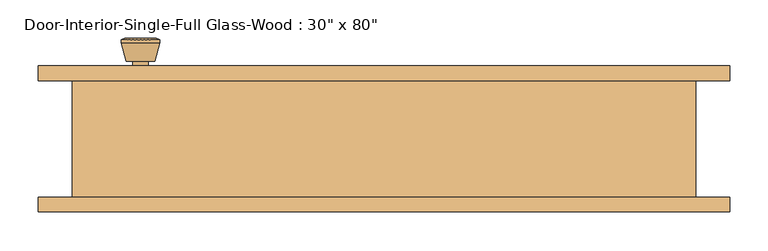
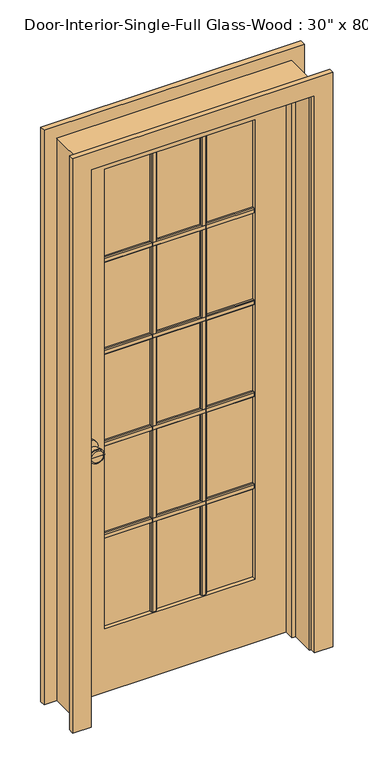
"""IFC4 building model written with IfcOpenShell, lengths in millimetres: door geometry."""

from ifc_helpers import new_model, si_unit, point, frame, frame_2d, origin, place, context, project, spatial, polyline, circle_curve, trimmed, segment, composite_curve, outline, extrude, faceted_brep, source, transform, mapped, element, save
from ifc_brep_helpers import plane_surface, cylinder_surface, revolved_surface, advanced_brep


def door_fa41f557(model_context):
    return source(origin(), model_context, "Body", "SolidModel", [
        extrude(outline(polyline([(59.055, 1586.23), (65.405, 1586.23), (68.58, 1583.055), (68.58, 1570.355), (65.405, 1567.18), (59.055, 1567.18), (59.055, 1586.23)])), frame((-260.35, 0.0, 0.0), z_axis=(1.0, 0.0, 0.0), x_axis=(0.0, 1.0, 0.0)), (0.0, 0.0, 1.0), 520.7),
        extrude(outline(polyline([(59.055, 1249.9975), (65.405, 1249.9975), (68.58, 1246.8225), (68.58, 1234.1225), (65.405, 1230.9475), (59.055, 1230.9475), (59.055, 1249.9975)])), frame((-260.35, 0.0, 0.0), z_axis=(1.0, 0.0, 0.0), x_axis=(0.0, 1.0, 0.0)), (0.0, 0.0, 1.0), 520.7),
        extrude(outline(polyline([(59.055, 913.765), (65.405, 913.765), (68.58, 910.59), (68.58, 897.89), (65.405, 894.715), (59.055, 894.715), (59.055, 913.765)])), frame((-260.35, 0.0, 0.0), z_axis=(1.0, 0.0, 0.0), x_axis=(0.0, 1.0, 0.0)), (0.0, 0.0, 1.0), 520.7),
        extrude(outline(polyline([(59.055, 577.5325), (65.405, 577.5325), (68.58, 574.3575), (68.58, 561.6575), (65.405, 558.4825), (59.055, 558.4825), (59.055, 577.5325)])), frame((-260.35, 0.0, 0.0), z_axis=(1.0, 0.0, 0.0), x_axis=(0.0, 1.0, 0.0)), (0.0, 0.0, 1.0), 520.7),
        extrude(outline(polyline([(77.2583333, 59.055), (77.2583333, 65.405), (80.4333333, 68.58), (93.1333333, 68.58), (96.3083333, 65.405), (96.3083333, 59.055), (77.2583333, 59.055)])), frame((0.0, 0.0, 231.775), z_axis=(0.0, 0.0, 1.0), x_axis=(1.0, 0.0, 0.0)), (0.0, 0.0, 1.0), 1681.1625),
        extrude(outline(polyline([(-96.3083333, 59.055), (-96.3083333, 65.405), (-93.1333333, 68.58), (-80.4333333, 68.58), (-77.2583333, 65.405), (-77.2583333, 59.055), (-96.3083333, 59.055)])), frame((0.0, 0.0, 231.775), z_axis=(0.0, 0.0, 1.0), x_axis=(1.0, 0.0, 0.0)), (0.0, 0.0, 1.0), 1681.1625),
        extrude(outline(polyline([(52.07, 1586.23), (52.07, 1567.18), (45.72, 1567.18), (42.545, 1570.355), (42.545, 1583.055), (45.72, 1586.23), (52.07, 1586.23)])), frame((-260.35, 0.0, 0.0), z_axis=(1.0, 0.0, 0.0), x_axis=(0.0, 1.0, 0.0)), (0.0, 0.0, 1.0), 520.7),
        extrude(outline(polyline([(52.07, 1249.9975), (52.07, 1230.9475), (45.72, 1230.9475), (42.545, 1234.1225), (42.545, 1246.8225), (45.72, 1249.9975), (52.07, 1249.9975)])), frame((-260.35, 0.0, 0.0), z_axis=(1.0, 0.0, 0.0), x_axis=(0.0, 1.0, 0.0)), (0.0, 0.0, 1.0), 520.7),
        extrude(outline(polyline([(52.07, 913.765), (52.07, 894.715), (45.72, 894.715), (42.545, 897.89), (42.545, 910.59), (45.72, 913.765), (52.07, 913.765)])), frame((-260.35, 0.0, 0.0), z_axis=(1.0, 0.0, 0.0), x_axis=(0.0, 1.0, 0.0)), (0.0, 0.0, 1.0), 520.7),
        extrude(outline(polyline([(52.07, 577.5325), (52.07, 558.4825), (45.72, 558.4825), (42.545, 561.6575), (42.545, 574.3575), (45.72, 577.5325), (52.07, 577.5325)])), frame((-260.35, 0.0, 0.0), z_axis=(1.0, 0.0, 0.0), x_axis=(0.0, 1.0, 0.0)), (0.0, 0.0, 1.0), 520.7),
        extrude(outline(polyline([(77.2583333, 52.07), (96.3083333, 52.07), (96.3083333, 45.72), (93.1333333, 42.545), (80.4333333, 42.545), (77.2583333, 45.72), (77.2583333, 52.07)])), frame((0.0, 0.0, 231.775), z_axis=(0.0, 0.0, 1.0), x_axis=(1.0, 0.0, 0.0)), (0.0, 0.0, 1.0), 1681.1625),
        extrude(outline(polyline([(-96.3083333, 52.07), (-77.2583333, 52.07), (-77.2583333, 45.72), (-80.4333333, 42.545), (-93.1333333, 42.545), (-96.3083333, 45.72), (-96.3083333, 52.07)])), frame((0.0, 0.0, 231.775), z_axis=(0.0, 0.0, 1.0), x_axis=(1.0, 0.0, 0.0)), (0.0, 0.0, 1.0), 1681.1625),
        advanced_brep(
        [(-317.5, 32.1, 914.4), (-307.5, 32.1, 914.4), (-327.5, 32.1, 914.4), (-297.0241324, -16.9, 914.4), (-317.5, -16.9, 914.4), (-337.9758676, -16.9, 914.4), (-292.5, -15.0721319, 914.4), (-342.5, -15.0721319, 914.4), (-292.5, -11.6084537, 914.4), (-342.5, -11.6084537, 914.4), (-298.863764, 13.1, 914.4), (-336.136236, 13.1, 914.4), (-307.5, 13.1, 914.4), (-327.5, 13.1, 914.4)],
        [
            (0, 1),
            (1, 2, circle_curve(frame((-317.5, 32.1, 914.4), z_axis=(0.0, 1.0, 0.0), x_axis=(-1.0, 0.0, 0.0)), 10.0)),
            (2, 0),
            (2, 1, circle_curve(frame((-317.5, 32.1, 914.4), z_axis=(0.0, 1.0, 0.0), x_axis=(-1.0, 0.0, 0.0)), 10.0)),
            (3, 4),
            (4, 5),
            (5, 3, circle_curve(frame((-317.5, -16.9, 914.4), z_axis=(0.0, -1.0, 0.0), x_axis=(-1.0, 0.0, 0.0)), 20.4758676)),
            (3, 5, circle_curve(frame((-317.5, -16.9, 914.4), z_axis=(0.0, -1.0, 0.0), x_axis=(-1.0, 0.0, 0.0)), 20.4758676)),
            (6, 3),
            (5, 7),
            (7, 6, circle_curve(frame((-317.5, -15.0721319, 914.4), z_axis=(0.0, -1.0, 0.0), x_axis=(-1.0, 0.0, 0.0)), 25.0)),
            (6, 7, circle_curve(frame((-317.5, -15.0721319, 914.4), z_axis=(0.0, -1.0, 0.0), x_axis=(-1.0, 0.0, 0.0)), 25.0)),
            (8, 6),
            (7, 9),
            (9, 8, circle_curve(frame((-317.5, -11.6084537, 914.4), z_axis=(0.0, -1.0, 0.0), x_axis=(-1.0, 0.0, 0.0)), 25.0)),
            (8, 9, circle_curve(frame((-317.5, -11.6084537, 914.4), z_axis=(0.0, -1.0, 0.0), x_axis=(-1.0, 0.0, 0.0)), 25.0)),
            (10, 8),
            (9, 11),
            (11, 10, circle_curve(frame((-317.5, 13.1, 914.4), z_axis=(0.0, -1.0, 0.0), x_axis=(-1.0, 0.0, 0.0)), 18.636236)),
            (10, 11, circle_curve(frame((-317.5, 13.1, 914.4), z_axis=(0.0, -1.0, 0.0), x_axis=(-1.0, 0.0, 0.0)), 18.636236)),
            (12, 10),
            (11, 13),
            (13, 12, circle_curve(frame((-317.5, 13.1, 914.4), z_axis=(0.0, -1.0, 0.0), x_axis=(-1.0, 0.0, 0.0)), 10.0)),
            (12, 13, circle_curve(frame((-317.5, 13.1, 914.4), z_axis=(0.0, -1.0, 0.0), x_axis=(-1.0, 0.0, 0.0)), 10.0)),
            (1, 12),
            (13, 2),
        ],
        [
            plane_surface(frame((-317.5, 32.1, 914.4), z_axis=(0.0, 1.0, 0.0), x_axis=(-1.0, 0.0, 0.0))),
            plane_surface(frame((-317.5, -16.9, 914.4), z_axis=(0.0, -1.0, 0.0), x_axis=(-1.0, 0.0, 0.0))),
            revolved_surface(polyline([(-337.9758676, -16.9, 914.4), (-342.5, -15.0721319, 914.4)]), (-317.5, 32.1, 914.4), (0.0, 1.0, 0.0)),
            cylinder_surface(frame((-317.5, 32.1, 914.4), z_axis=(0.0, 1.0, 0.0), x_axis=(-1.0, 0.0, 0.0)), 25.0),
            revolved_surface(polyline([(-342.5, -11.6084537, 914.4), (-336.136236, 13.1, 914.4)]), (-317.5, 32.1, 914.4), (0.0, 1.0, 0.0)),
            plane_surface(frame((-317.5, 13.1, 914.4), z_axis=(0.0, 1.0, 0.0), x_axis=(-1.0, 0.0, 0.0))),
            cylinder_surface(frame((-317.5, 32.1, 914.4), z_axis=(0.0, 1.0, 0.0), x_axis=(-1.0, 0.0, 0.0)), 10.0),
        ],
        [
            (0, [[1, 2, 3]]),
            (0, [[-3, 4, -1]]),
            (1, [[5, 6, 7]]),
            (1, [[-6, -5, 8]]),
            (2, [[9, -7, 10, 11]]),
            (2, [[-10, -8, -9, 12]]),
            (3, [[13, -11, 14, 15]]),
            (3, [[-14, -12, -13, 16]]),
            (4, [[17, -15, 18, 19]]),
            (4, [[-18, -16, -17, 20]]),
            (5, [[21, -19, 22, 23]]),
            (5, [[-22, -20, -21, 24]]),
            (6, [[25, -23, 26, -2]]),
            (6, [[-26, -24, -25, -4]]),
        ],
    ),
        extrude(outline(composite_curve([segment(trimmed(circle_curve(frame_2d((914.4, -317.5)), 30.0), [point((914.4, -347.5))], [point((914.4, -287.5))], False, "CARTESIAN"), True, "CONTINUOUS"), segment(trimmed(circle_curve(frame_2d((914.4, -317.5)), 30.0), [point((914.4, -287.5))], [point((914.4, -347.5))], False, "CARTESIAN"), True, "CONTINUOUS")], self_intersect=False)), frame((0.0, 32.1, 0.0), z_axis=(0.0, 1.0, 0.0), x_axis=(0.0, 0.0, 1.0)), (0.0, 0.0, 1.0), 6.0),
        advanced_brep(
        [(-317.5, 79.025, 914.4), (-327.5, 79.025, 914.4), (-307.5, 79.025, 914.4), (-297.0241324, 128.025, 914.4), (-337.9758676, 128.025, 914.4), (-317.5, 128.025, 914.4), (-292.5, 126.1971319, 914.4), (-342.5, 126.1971319, 914.4), (-292.5, 122.7334537, 914.4), (-342.5, 122.7334537, 914.4), (-298.863764, 98.025, 914.4), (-336.136236, 98.025, 914.4), (-307.5, 98.025, 914.4), (-327.5, 98.025, 914.4)],
        [
            (0, 1),
            (1, 2, circle_curve(frame((-317.5, 79.025, 914.4), z_axis=(0.0, -1.0, 0.0), x_axis=(-1.0, 0.0, 0.0)), 10.0)),
            (2, 0),
            (2, 1, circle_curve(frame((-317.5, 79.025, 914.4), z_axis=(0.0, -1.0, 0.0), x_axis=(-1.0, 0.0, 0.0)), 10.0)),
            (3, 4, circle_curve(frame((-317.5, 128.025, 914.4), z_axis=(0.0, 1.0, 0.0), x_axis=(-1.0, 0.0, 0.0)), 20.4758676)),
            (4, 5),
            (5, 3),
            (4, 3, circle_curve(frame((-317.5, 128.025, 914.4), z_axis=(0.0, 1.0, 0.0), x_axis=(-1.0, 0.0, 0.0)), 20.4758676)),
            (6, 7, circle_curve(frame((-317.5, 126.1971319, 914.4), z_axis=(0.0, 1.0, 0.0), x_axis=(-1.0, 0.0, 0.0)), 25.0)),
            (7, 4),
            (3, 6),
            (7, 6, circle_curve(frame((-317.5, 126.1971319, 914.4), z_axis=(0.0, 1.0, 0.0), x_axis=(-1.0, 0.0, 0.0)), 25.0)),
            (8, 9, circle_curve(frame((-317.5, 122.7334537, 914.4), z_axis=(0.0, 1.0, 0.0), x_axis=(-1.0, 0.0, 0.0)), 25.0)),
            (9, 7),
            (6, 8),
            (9, 8, circle_curve(frame((-317.5, 122.7334537, 914.4), z_axis=(0.0, 1.0, 0.0), x_axis=(-1.0, 0.0, 0.0)), 25.0)),
            (10, 11, circle_curve(frame((-317.5, 98.025, 914.4), z_axis=(0.0, 1.0, 0.0), x_axis=(-1.0, 0.0, 0.0)), 18.636236)),
            (11, 9),
            (8, 10),
            (11, 10, circle_curve(frame((-317.5, 98.025, 914.4), z_axis=(0.0, 1.0, 0.0), x_axis=(-1.0, 0.0, 0.0)), 18.636236)),
            (12, 13, circle_curve(frame((-317.5, 98.025, 914.4), z_axis=(0.0, 1.0, 0.0), x_axis=(-1.0, 0.0, 0.0)), 10.0)),
            (13, 11),
            (10, 12),
            (13, 12, circle_curve(frame((-317.5, 98.025, 914.4), z_axis=(0.0, 1.0, 0.0), x_axis=(-1.0, 0.0, 0.0)), 10.0)),
            (1, 13),
            (12, 2),
        ],
        [
            plane_surface(frame((-317.5, 79.025, 914.4), z_axis=(0.0, -1.0, 0.0), x_axis=(-1.0, 0.0, 0.0))),
            plane_surface(frame((-317.5, 128.025, 914.4), z_axis=(0.0, 1.0, 0.0), x_axis=(-1.0, 0.0, 0.0))),
            revolved_surface(polyline([(-337.9758676, 128.025, 914.4), (-342.5, 126.1971319, 914.4)]), (-317.5, 79.025, 914.4), (0.0, -1.0, 0.0)),
            cylinder_surface(frame((-317.5, 79.025, 914.4), z_axis=(0.0, -1.0, 0.0), x_axis=(-1.0, 0.0, 0.0)), 25.0),
            revolved_surface(polyline([(-342.5, 122.7334537, 914.4), (-336.136236, 98.025, 914.4)]), (-317.5, 79.025, 914.4), (0.0, -1.0, 0.0)),
            plane_surface(frame((-317.5, 98.025, 914.4), z_axis=(0.0, -1.0, 0.0), x_axis=(-1.0, 0.0, 0.0))),
            cylinder_surface(frame((-317.5, 79.025, 914.4), z_axis=(0.0, -1.0, 0.0), x_axis=(-1.0, 0.0, 0.0)), 10.0),
        ],
        [
            (0, [[1, 2, 3]]),
            (0, [[-3, 4, -1]]),
            (1, [[5, 6, 7]]),
            (1, [[8, -7, -6]]),
            (2, [[9, 10, -5, 11]]),
            (2, [[12, -11, -8, -10]]),
            (3, [[13, 14, -9, 15]]),
            (3, [[16, -15, -12, -14]]),
            (4, [[17, 18, -13, 19]]),
            (4, [[20, -19, -16, -18]]),
            (5, [[21, 22, -17, 23]]),
            (5, [[24, -23, -20, -22]]),
            (6, [[-2, 25, -21, 26]]),
            (6, [[-4, -26, -24, -25]]),
        ],
    ),
        extrude(outline(composite_curve([segment(trimmed(circle_curve(frame_2d((914.4, -317.5)), 30.0), [point((914.4, -347.5))], [point((914.4, -287.5))], False, "CARTESIAN"), True, "CONTINUOUS"), segment(trimmed(circle_curve(frame_2d((914.4, -317.5)), 30.0), [point((914.4, -287.5))], [point((914.4, -347.5))], False, "CARTESIAN"), True, "CONTINUOUS")], self_intersect=False)), frame((0.0, 73.025, 0.0), z_axis=(0.0, 1.0, 0.0), x_axis=(0.0, 0.0, 1.0)), (0.0, 0.0, 1.0), 6.0),
        extrude(outline(polyline([(2032.0, -381.0), (0.0, -381.0), (0.0, 381.0), (2032.0, 381.0), (2032.0, -381.0)]), holes=[polyline([(1912.9375, -260.35), (1912.9375, 260.35), (231.775, 260.35), (231.775, -260.35), (1912.9375, -260.35)])]), frame((0.0, 38.1, 0.0), z_axis=(0.0, 1.0, 0.0), x_axis=(0.0, 0.0, 1.0)), (0.0, 0.0, 1.0), 34.925),
        faceted_brep([(406.4, 73.025, 0.0), (406.4, -79.375, 0.0), (381.0, -79.375, 0.0), (381.0, 3.175, 0.0), (368.3, 3.175, 0.0), (368.3, 38.1, 0.0), (381.0, 38.1, 0.0), (381.0, 73.025, 0.0), (406.4, 73.025, 2057.4), (406.4, -79.375, 2057.4), (-406.4, -79.375, 2057.4), (-406.4, -79.375, 0.0), (-381.0, -79.375, 0.0), (-381.0, -79.375, 2032.0), (381.0, -79.375, 2032.0), (381.0, 3.175, 2032.0), (-381.0, 3.175, 2032.0), (-381.0, 3.175, 0.0), (-368.3, 3.175, 0.0), (-368.3, 3.175, 2019.3), (368.3, 3.175, 2019.3), (368.3, 38.1, 2019.3), (-368.3, 38.1, 2019.3), (-368.3, 38.1, 0.0), (-381.0, 38.1, 0.0), (-381.0, 38.1, 2032.0), (381.0, 38.1, 2032.0), (381.0, 73.025, 2032.0), (-381.0, 73.025, 2032.0), (-381.0, 73.025, 0.0), (-406.4, 73.025, 0.0), (-406.4, 73.025, 2057.4)], [[[0, 1, 2, 3, 4, 5, 6, 7]], [[1, 0, 8, 9]], [[2, 1, 9, 10, 11, 12, 13, 14]], [[3, 2, 14, 15]], [[4, 3, 15, 16, 17, 18, 19, 20]], [[5, 4, 20, 21]], [[6, 5, 21, 22, 23, 24, 25, 26]], [[7, 6, 26, 27]], [[0, 7, 27, 28, 29, 30, 31, 8]], [[9, 8, 31, 10]], [[15, 14, 13, 16]], [[21, 20, 19, 22]], [[27, 26, 25, 28]], [[30, 29, 24, 23, 18, 17, 12, 11]], [[10, 31, 30, 11]], [[16, 13, 12, 17]], [[22, 19, 18, 23]], [[28, 25, 24, 29]]]),
        extrude(outline(polyline([(260.35, 52.07), (-260.35, 52.07), (-260.35, 59.055), (260.35, 59.055), (260.35, 52.07)])), frame((0.0, 0.0, 231.775), z_axis=(0.0, 0.0, 1.0), x_axis=(1.0, 0.0, 0.0)), (0.0, 0.0, 1.0), 1681.1625),
        extrude(outline(polyline([(0.0, 387.35), (0.0, 450.85), (2101.85, 450.85), (2101.85, -450.85), (0.0, -450.85), (0.0, -387.35), (2038.35, -387.35), (2038.35, 387.35), (0.0, 387.35)])), frame((0.0, -98.425, 0.0), z_axis=(0.0, 1.0, 0.0), x_axis=(0.0, 0.0, 1.0)), (0.0, 0.0, 1.0), 19.05),
        extrude(outline(polyline([(0.0, 387.35), (0.0, 450.85), (2101.85, 450.85), (2101.85, -450.85), (0.0, -450.85), (0.0, -387.35), (2038.35, -387.35), (2038.35, 387.35), (0.0, 387.35)])), frame((0.0, 73.025, 0.0), z_axis=(0.0, 1.0, 0.0), x_axis=(0.0, 0.0, 1.0)), (0.0, 0.0, 1.0), 19.05),
    ])


if __name__ == "__main__":
    model = new_model("IFC4")
    model_context = context("Model", 3, world=origin())
    ifc_project = project(units=[si_unit("LENGTHUNIT", "METRE", prefix="MILLI")], contexts=[model_context])
    site = spatial("IfcSite", under=ifc_project)
    building = spatial("IfcBuilding", under=site)
    placement = place(None, origin())
    door_shape = door_fa41f557(model_context)
    element("IfcDoor", 1, ObjectType="Door-Interior-Single-Full Glass-Wood : 30\" x 80\"", at=placement, inside=building, context=model_context, shape_type="MappedRepresentation", body=[
        mapped(door_shape, transform((0.0, 0.0, 0.0), x_axis=(1.0, 0.0, 0.0), y_axis=(0.0, 1.0, 0.0), z_axis=(0.0, 0.0, 1.0))),
    ])
    save(model, "model.ifc")

# Revit data of these elements
# Type "Door-Interior-Single-Full Glass-Wood : 30\" x 80\""
#   Type Mark = "11"
#   Assembly Code = "C1020300"
#   Analytic Construction = "Wood frame with single clear glass"
#   Top Rail = 0' - 4 11/16"
#   Thickness = 0' - 1 3/8"
#   Thermal Resistance (R) = 1.0102 (h·ft²·°F)/BTU
#   Swing Angle [instance default] = 90.00°
#   Stiles = 0' - 4 3/4"
#   Rough Width = 2' - 8"
#   Rough Height = 6' - 9"
#   Height = 6' - 8"
#   Width = 2' - 6"
#   Heat Transfer Coefficient (U) = 0.9900 BTU/(h·ft²·°F)
#   Bottom Rail = 0' - 9 1/8"
#   Show Grill [instance default] = yes
#   Trim Material = Cherry
#   Panel Material = Cherry
#   Frame Material = Cherry
#   Door Handle Material = Aluminum
#   Visual Light Transmittance = 0
#   Solar Heat Gain Coefficient = 0
#   Wall Closure = (empty or 0)
#   Function = (empty or 0)
# Element 1 (IfcDoor, "Door-Interior-Single-Full Glass-Wood : 30\" x 80\"")
#   Materials on its faces: "Cherry", "Aluminum", "Glass"
# Materials
#   "Cherry": class "Wood", colour RGB 226 177 128, transparency 0, Description = "Prunus Serotina", Cost = 0
#   "Aluminum": class "Metal", colour RGB 247 247 247, transparency 0, Description = "Aluminum 6061", Cost = 0
#   "Glass": class "Glass", colour RGB 0 128 192, transparency 0.75, Description = "Soda Lime Glass", Cost = 0
